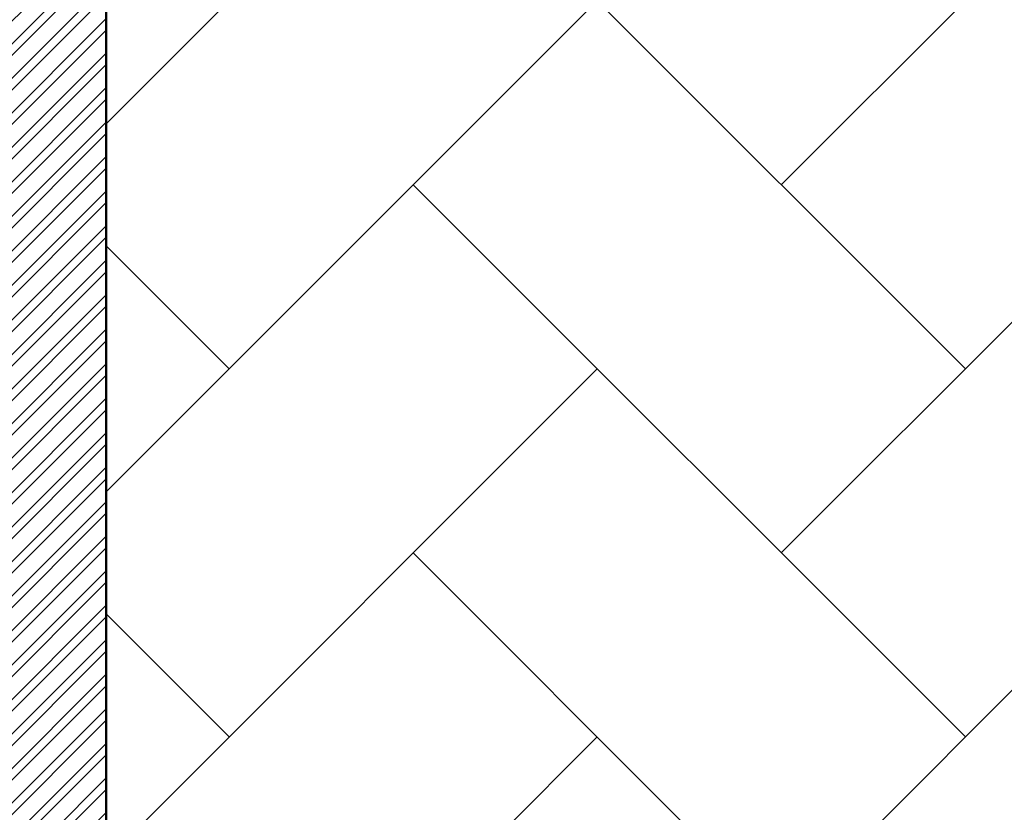
# Model space of a CAD drawing. Units: inches. Extents: x 3590 to 5167, y 65 to 1917.
# Tile 36 of 100: x 4927 to 5003, y 1388 to 1450. Entities that reach past the tile are written whole.
import ezdxf

# ---------------------------------------------------------------- set-up
doc = ezdxf.new("R2010")
doc.units = ezdxf.units.IN
for name, color, linetype, lineweight in [('A-FLOR-PATT', 8, 'Continuous', 13), ('A-WALL', 7, 'Continuous', 50), ('A-WALL-PATT', 251, 'Continuous', 13)]:
    doc.layers.add(name, color=color, linetype=linetype, lineweight=lineweight)

msp = doc.modelspace()

# ---------------------------------------------------------------- hatches: boundary and pattern name
at = {"layer": 'A-FLOR-PATT', "transparency": 33554687}
h = msp.add_hatch(dxfattribs=at)
h.set_pattern_fill('AR-HBONE', color=256, scale=0.2)
h.set_pattern_definition([(45, (-588.972, 0), (0, 28.73682), [60.96, -20.32]), (135, (-574.604, 14.368), (3e-15, 28.73682), [60.96, -20.32])])
h.paths.add_polyline_path([(5071.274, 1796.999), (4933.274, 1796.999), (4933.274, 1753.999), (4962.774, 1753.999, -0.414214), (4928.774, 1719.999), (4933.274, 1718.999), (4933.274, 1334.999), (5071.274, 1334.999)])
h.paths.add_polyline_path([(4951.78, 1521.077), (4951.715, 1521.04), (4951.563, 1520.895)], flags=16)
h.paths.add_polyline_path([(4952.267, 1521.376), (4952.198, 1521.371), (4952.198, 1521.356)], flags=0)
h.paths.add_polyline_path([(4967.051, 1529.728), (4965.231, 1528.694), (4963.411, 1527.714), (4961.756, 1526.851), (4963.589, 1527.449), (4964.036, 1527.478), (4962.975, 1527.249), (4961.76, 1526.852), (4959.792, 1525.834), (4958.005, 1524.895), (4956.24, 1523.93), (4954.504, 1522.919), (4954.129, 1522.682), (4953.361, 1521.997), (4953.366, 1521.998), (4953.605, 1522.064), (4955.106, 1522.761), (4956.921, 1523.434), (4958.678, 1523.915), (4960.358, 1524.2), (4961.945, 1524.286), (4964.171, 1524.108), (4965.958, 1523.309), (4963.863, 1522.976), (4965.187, 1522.499), (4963.366, 1522.497), (4961.545, 1522.487), (4959.764, 1522.461), (4958.304, 1522.419), (4957.974, 1522.388), (4956.307, 1522.232), (4954.718, 1522.071), (4953.251, 1521.899), (4953.525, 1521.623), (4954.331, 1521.379), (4956.243, 1521.23), (4958.039, 1520.93), (4959.684, 1520.483), (4961.16, 1519.896), (4963.107, 1518.8), (4964.393, 1517.325), (4962.973, 1517.726), (4964.558, 1516.661), (4965.407, 1515.708), (4963.507, 1516.322), (4961.68, 1517.005), (4959.935, 1517.745), (4958.282, 1518.528), (4956.732, 1519.343), (4955.295, 1520.175), (4954.672, 1520.572), (4954.513, 1520.627), (4955.658, 1519.318), (4956.703, 1517.982), (4957.644, 1516.647), (4958.485, 1515.334), (4959.55, 1513.524), (4960.438, 1511.769), (4958.841, 1513.62), (4957.452, 1515.325), (4955.819, 1517.459), (4956.665, 1515.448), (4957.111, 1513.923), (4957.447, 1511.714), (4957.076, 1509.793), (4956.538, 1511.11), (4955.992, 1512.569), (4955.444, 1514.125), (4954.898, 1515.735), (4954.357, 1517.356), (4953.824, 1518.943), (4953.305, 1520.452), (4953.065, 1521.116), (4952.971, 1521.146), (4952.949, 1521.086), (4952.73, 1520.199), (4953.37, 1518.024), (4953.757, 1516.373), (4954.051, 1514.765), (4954.264, 1513.221), (4954.471, 1511.131), (4954.497, 1510.402), (4954.409, 1511.76), (4954.264, 1513.221), (4954.051, 1514.765), (4953.757, 1516.373), (4953.37, 1518.024), (4952.877, 1519.698), (4952.716, 1520.141), (4952.533, 1519.059), (4952.374, 1517.789), (4952.219, 1516.312), (4952.046, 1514.6), (4951.833, 1512.626), (4951.557, 1510.363), (4951.203, 1512.168), (4950.852, 1514.339), (4950.985, 1516.376), (4951.66, 1518.286), (4952.593, 1520.481), (4952.357, 1521.13), (4951.855, 1520.328), (4950.839, 1518.908), (4949.777, 1517.587), (4948.916, 1516.617), (4948.111, 1515.256), (4947.089, 1513.554), (4945.889, 1511.615), (4946.326, 1513.402), (4946.562, 1514.249), (4945.528, 1513.327), (4944.581, 1512.531), (4946.018, 1514.508), (4947.204, 1516.048), (4947.893, 1517.313), (4949.307, 1518.764), (4950.414, 1519.767), (4950.451, 1519.806), (4952.267, 1521.376), (4951.645, 1521.493), (4950.404, 1521.18), (4948.044, 1520.359), (4946.119, 1519.452), (4944.572, 1518.475), (4943.35, 1517.443), (4941.997, 1515.92), (4941.661, 1515.275), (4942.813, 1516.99), (4944.572, 1518.475), (4946.119, 1519.452), (4948.044, 1520.359), (4950.404, 1521.18), (4951.645, 1521.493), (4949.647, 1521.868), (4948.6, 1521.756), (4947.126, 1521.57), (4945.42, 1521.348), (4943.45, 1521.105), (4941.183, 1520.856), (4942.86, 1521.613), (4943.873, 1522.03), (4942.952, 1521.909), (4941.41, 1521.485), (4939.543, 1520.67), (4938.968, 1520.226), (4940.733, 1521.299), (4942.952, 1521.909), (4943.702, 1522.008), (4945.894, 1522.7), (4947.565, 1522.714), (4948.921, 1522.566), (4951.131, 1522.183), (4950.971, 1522.297), (4948.129, 1523.006), (4946.035, 1523.707), (4944.232, 1524.521), (4942.707, 1525.461), (4941.444, 1526.537), (4940.43, 1527.761), (4939.649, 1529.143), (4941.421, 1528.122), (4943.147, 1527.132), (4944.841, 1526.175), (4946.514, 1525.25), (4948.179, 1524.359), (4948.365, 1524.263), (4946.475, 1526.045), (4945.181, 1527.54), (4944.19, 1529.033), (4943.496, 1530.54), (4943.278, 1531.36), (4942.498, 1531.919), (4943.114, 1531.762), (4942.959, 1533.659), (4944.14, 1531.989), (4944.612, 1531.323), (4946.202, 1530.463), (4947.486, 1529.509), (4948.79, 1528.226), (4950.368, 1526.237), (4949.485, 1528.155), (4948.851, 1530.123), (4948.491, 1532.041), (4948.381, 1533.918), (4948.501, 1535.76), (4948.827, 1537.573), (4949.418, 1535.565), (4949.957, 1533.569), (4950.464, 1531.586), (4950.961, 1529.617), (4951.391, 1527.954), (4951.724, 1530.687), (4952.201, 1532.58), (4952.889, 1534.33), (4953.77, 1535.951), (4954.827, 1537.46), (4954.521, 1535.39), (4954.273, 1533.937), (4955.58, 1535.663), (4956.748, 1536.739), (4956.159, 1534.78), (4955.589, 1532.873), (4955.043, 1531.006), (4954.525, 1529.166), (4954.038, 1527.341), (4953.638, 1525.733), (4953.611, 1525.586), (4953.398, 1524.166), (4953.382, 1524.009), (4954.07, 1525.476), (4954.912, 1527.022), (4956.136, 1528.894), (4957.847, 1530.577), (4959.376, 1531.54), (4958.256, 1530.104), (4957.143, 1528.663), (4956.066, 1527.243), (4955.056, 1525.871), (4954.141, 1524.571), (4953.352, 1523.372), (4953.311, 1523.303), (4953.273, 1522.925), (4953.261, 1522.382), (4954.103, 1523.373), (4954.63, 1524.284), (4955.961, 1526.358), (4957.23, 1528.13), (4958.421, 1529.609), (4960.037, 1531.368), (4961.374, 1532.375), (4962.101, 1532.77), (4961.07, 1531.061), (4959.987, 1529.438), (4958.869, 1527.908), (4958.15, 1527.007), (4959.803, 1528.003), (4961.589, 1528.793), (4963.391, 1529.328), (4965.211, 1529.632)], flags=16)
h.paths.add_polyline_path([(4962.944, 1523.182), (4961.107, 1523.422), (4960.392, 1523.362), (4962.35, 1523.331)], flags=0)
h.paths.add_polyline_path([(5049.541, 1584.551), (5049.476, 1584.515), (5049.325, 1584.37)], flags=16)
h.paths.add_polyline_path([(5050.028, 1584.851), (5049.959, 1584.845), (5049.959, 1584.83)], flags=0)
h.paths.add_polyline_path([(5042.333, 1581.949), (5043.88, 1582.926), (5045.806, 1583.833), (5048.165, 1584.654), (5049.406, 1584.967), (5047.408, 1585.342), (5046.361, 1585.231), (5044.888, 1585.044), (5043.181, 1584.822), (5041.211, 1584.579), (5038.944, 1584.33), (5040.622, 1585.087), (5041.634, 1585.504), (5040.713, 1585.383), (5039.171, 1584.959), (5037.304, 1584.144), (5036.729, 1583.7), (5038.494, 1584.773), (5040.713, 1585.383), (5041.463, 1585.482), (5043.655, 1586.174), (5045.326, 1586.188), (5046.682, 1586.04), (5048.893, 1585.657), (5048.732, 1585.771), (5045.891, 1586.48), (5043.796, 1587.181), (5041.994, 1587.996), (5040.468, 1588.935), (5039.205, 1590.011), (5038.191, 1591.235), (5037.41, 1592.617), (5039.182, 1591.596), (5040.909, 1590.607), (5042.602, 1589.649), (5044.275, 1588.724), (5045.94, 1587.833), (5046.126, 1587.738), (5044.237, 1589.519), (5042.942, 1591.015), (5041.952, 1592.508), (5041.257, 1594.014), (5041.039, 1594.834), (5040.26, 1595.393), (5040.875, 1595.237), (5040.721, 1597.133), (5041.901, 1595.463), (5042.373, 1594.798), (5043.963, 1593.938), (5045.247, 1592.983), (5046.552, 1591.701), (5048.129, 1589.712), (5047.247, 1591.63), (5046.613, 1593.597), (5046.252, 1595.515), (5046.142, 1597.392), (5046.262, 1599.234), (5046.588, 1601.047), (5047.179, 1599.039), (5047.718, 1597.043), (5048.225, 1595.06), (5048.722, 1593.091), (5049.152, 1591.429), (5049.485, 1594.161), (5049.962, 1596.054), (5050.65, 1597.804), (5051.532, 1599.425), (5052.589, 1600.934), (5052.283, 1598.864), (5052.034, 1597.411), (5053.341, 1599.137), (5054.509, 1600.213), (5053.92, 1598.254), (5053.35, 1596.348), (5052.805, 1594.48), (5052.286, 1592.64), (5051.799, 1590.815), (5051.4, 1589.207), (5051.373, 1589.06), (5051.159, 1587.64), (5051.143, 1587.483), (5051.831, 1588.95), (5052.673, 1590.496), (5053.898, 1592.368), (5055.608, 1594.051), (5057.137, 1595.014), (5056.017, 1593.578), (5054.904, 1592.137), (5053.828, 1590.717), (5052.817, 1589.345), (5051.902, 1588.046), (5051.113, 1586.846), (5051.072, 1586.777), (5051.034, 1586.399), (5051.022, 1585.856), (5051.864, 1586.847), (5052.391, 1587.758), (5053.723, 1589.832), (5054.991, 1591.604), (5056.182, 1593.083), (5057.798, 1594.842), (5059.135, 1595.849), (5059.863, 1596.244), (5058.831, 1594.535), (5057.749, 1592.912), (5056.63, 1591.382), (5055.912, 1590.482), (5057.564, 1591.477), (5059.35, 1592.267), (5061.152, 1592.802), (5062.972, 1593.106), (5064.812, 1593.203), (5062.992, 1592.169), (5061.172, 1591.188), (5059.518, 1590.325), (5061.35, 1590.924), (5061.797, 1590.952), (5060.737, 1590.723), (5059.521, 1590.326), (5057.553, 1589.308), (5055.766, 1588.369), (5054.002, 1587.404), (5052.265, 1586.393), (5051.891, 1586.156), (5051.122, 1585.471), (5051.127, 1585.472), (5051.366, 1585.538), (5052.867, 1586.235), (5054.682, 1586.908), (5056.439, 1587.389), (5058.12, 1587.675), (5059.706, 1587.76), (5061.933, 1587.583), (5063.719, 1586.783), (5061.624, 1586.45), (5062.949, 1585.973), (5061.127, 1585.971), (5059.307, 1585.961), (5057.525, 1585.935), (5056.065, 1585.893), (5055.735, 1585.862), (5054.068, 1585.707), (5052.479, 1585.546), (5051.012, 1585.373), (5051.286, 1585.097), (5052.092, 1584.853), (5054.004, 1584.704), (5055.8, 1584.404), (5057.446, 1583.958), (5058.921, 1583.37), (5060.868, 1582.274), (5062.154, 1580.799), (5060.734, 1581.2), (5062.32, 1580.135), (5063.168, 1579.182), (5061.269, 1579.796), (5059.441, 1580.479), (5057.696, 1581.219), (5056.043, 1582.003), (5054.493, 1582.817), (5053.057, 1583.649), (5052.433, 1584.047), (5052.274, 1584.101), (5053.42, 1582.793), (5054.464, 1581.457), (5055.405, 1580.121), (5056.247, 1578.809), (5057.311, 1576.998), (5058.199, 1575.244), (5056.602, 1577.094), (5055.213, 1578.799), (5053.58, 1580.933), (5054.427, 1578.922), (5054.872, 1577.397), (5055.208, 1575.189), (5054.838, 1573.267), (5054.299, 1574.584), (5053.754, 1576.043), (5053.206, 1577.599), (5052.659, 1579.209), (5052.118, 1580.83), (5051.585, 1582.417), (5051.066, 1583.927), (5050.826, 1584.59), (5050.733, 1584.62), (5050.711, 1584.561), (5050.491, 1583.673), (5051.131, 1581.498), (5051.518, 1579.847), (5051.813, 1578.24), (5052.026, 1576.695), (5052.233, 1574.605), (5052.258, 1573.876), (5052.17, 1575.234), (5052.026, 1576.695), (5051.813, 1578.24), (5051.518, 1579.847), (5051.131, 1581.498), (5050.638, 1583.172), (5050.477, 1583.615), (5050.294, 1582.533), (5050.136, 1581.263), (5049.981, 1579.786), (5049.807, 1578.074), (5049.594, 1576.1), (5049.318, 1573.837), (5048.965, 1575.642), (5048.613, 1577.813), (5048.747, 1579.85), (5049.421, 1581.76), (5050.354, 1583.955), (5050.118, 1584.604), (5049.616, 1583.802), (5048.6, 1582.382), (5047.538, 1581.061), (5046.677, 1580.091), (5045.872, 1578.73), (5044.85, 1577.028), (5043.651, 1575.089), (5044.087, 1576.877), (5044.324, 1577.723), (5043.289, 1576.801), (5042.342, 1576.005), (5043.779, 1577.982), (5044.966, 1579.522), (5045.655, 1580.787), (5047.068, 1582.239), (5048.175, 1583.241), (5048.213, 1583.28), (5050.028, 1584.851), (5049.406, 1584.967), (5048.165, 1584.654), (5045.806, 1583.833), (5043.88, 1582.926), (5042.333, 1581.949), (5041.111, 1580.917), (5039.758, 1579.394), (5039.423, 1578.749), (5040.575, 1580.464)], flags=16)
h.paths.add_polyline_path([(4954.799, 1533.12), (4954.262, 1532.079), (4953.831, 1530.935), (4953.505, 1529.636), (4953.283, 1528.133), (4953.167, 1526.376), (4953.156, 1524.315), (4953.277, 1521.236), (4952.802, 1521.842), (4951.557, 1521.998), (4950.976, 1521.961), (4952.661, 1521.941), (4952.802, 1521.842), (4953.152, 1523.593), (4953.167, 1526.376), (4953.283, 1528.133), (4953.609, 1530.346), (4954.456, 1532.592)], flags=0)
h.paths.add_polyline_path([(5050.563, 1585.316), (5049.318, 1585.472), (5048.737, 1585.435), (5050.422, 1585.415), (5050.563, 1585.316), (5050.914, 1587.067), (5050.928, 1589.851), (5051.045, 1591.607), (5051.371, 1593.82), (5052.217, 1596.066), (5052.56, 1596.594), (5052.024, 1595.554), (5051.592, 1594.409), (5051.266, 1593.11), (5051.045, 1591.607), (5050.928, 1589.851), (5050.918, 1587.789), (5051.038, 1584.71)], flags=0)
h.paths.add_polyline_path([(5058.153, 1586.836), (5060.111, 1586.805), (5060.705, 1586.656), (5058.868, 1586.896)], flags=0)
h.paths.add_polyline_path([(5049.541, 1430.936), (5049.476, 1430.9), (5049.325, 1430.755)], flags=16)
h.paths.add_polyline_path([(5050.028, 1431.236), (5049.959, 1431.231), (5049.959, 1431.215)], flags=0)
h.paths.add_polyline_path([(5046.588, 1447.432), (5047.179, 1445.425), (5047.718, 1443.429), (5048.225, 1441.446), (5048.722, 1439.476), (5049.152, 1437.814), (5049.485, 1440.546), (5049.962, 1442.439), (5050.65, 1444.189), (5051.532, 1445.811), (5052.589, 1447.319), (5052.283, 1445.249), (5052.034, 1443.796), (5053.341, 1445.522), (5054.509, 1446.598), (5053.92, 1444.64), (5053.35, 1442.733), (5052.805, 1440.865), (5052.286, 1439.025), (5051.799, 1437.201), (5051.4, 1435.592), (5051.373, 1435.445), (5051.159, 1434.025), (5051.143, 1433.868), (5051.831, 1435.335), (5052.673, 1436.881), (5053.898, 1438.753), (5055.608, 1440.436), (5057.137, 1441.4), (5056.017, 1439.963), (5054.904, 1438.522), (5053.828, 1437.102), (5052.817, 1435.73), (5051.902, 1434.431), (5051.113, 1433.231), (5051.072, 1433.162), (5051.034, 1432.784), (5051.022, 1432.242), (5051.864, 1433.232), (5052.391, 1434.143), (5053.723, 1436.217), (5054.991, 1437.989), (5056.182, 1439.468), (5057.798, 1441.227), (5059.135, 1442.235), (5059.863, 1442.629), (5058.831, 1440.921), (5057.749, 1439.298), (5056.63, 1437.767), (5055.912, 1436.867), (5057.564, 1437.863), (5059.35, 1438.652), (5061.152, 1439.187), (5062.972, 1439.491), (5064.812, 1439.588), (5062.992, 1438.554), (5061.172, 1437.573), (5059.518, 1436.71), (5061.35, 1437.309), (5061.797, 1437.337), (5060.737, 1437.108), (5059.521, 1436.711), (5057.553, 1435.693), (5055.766, 1434.754), (5054.002, 1433.789), (5052.265, 1432.778), (5051.891, 1432.541), (5051.122, 1431.856), (5051.127, 1431.857), (5051.366, 1431.923), (5052.867, 1432.62), (5054.682, 1433.293), (5056.439, 1433.775), (5058.12, 1434.06), (5059.706, 1434.145), (5061.933, 1433.968), (5063.719, 1433.168), (5061.624, 1432.835), (5062.949, 1432.358), (5061.127, 1432.357), (5059.307, 1432.346), (5057.525, 1432.32), (5056.065, 1432.278), (5055.735, 1432.248), (5054.068, 1432.092), (5052.479, 1431.931), (5051.012, 1431.759), (5051.286, 1431.482), (5052.092, 1431.238), (5054.004, 1431.089), (5055.8, 1430.789), (5057.446, 1430.343), (5058.921, 1429.755), (5060.868, 1428.66), (5062.154, 1427.185), (5060.734, 1427.585), (5062.32, 1426.52), (5063.168, 1425.567), (5061.269, 1426.181), (5059.441, 1426.865), (5057.696, 1427.604), (5056.043, 1428.388), (5054.493, 1429.202), (5053.057, 1430.034), (5052.433, 1430.432), (5052.274, 1430.487), (5053.42, 1429.178), (5054.464, 1427.842), (5055.405, 1426.506), (5056.247, 1425.194), (5057.311, 1423.383), (5058.199, 1421.629), (5056.602, 1423.479), (5055.213, 1425.184), (5053.58, 1427.318), (5054.427, 1425.307), (5054.872, 1423.782), (5055.208, 1421.574), (5054.838, 1419.652), (5054.299, 1420.97), (5053.754, 1422.428), (5053.206, 1423.984), (5052.659, 1425.595), (5052.118, 1427.215), (5051.585, 1428.802), (5051.066, 1430.312), (5050.826, 1430.975), (5050.733, 1431.005), (5050.711, 1430.946), (5050.491, 1430.058), (5051.131, 1427.883), (5051.518, 1426.232), (5051.813, 1424.625), (5052.026, 1423.081), (5052.233, 1420.991), (5052.258, 1420.261), (5052.17, 1421.619), (5052.026, 1423.081), (5051.813, 1424.625), (5051.518, 1426.232), (5051.131, 1427.883), (5050.638, 1429.558), (5050.477, 1430.001), (5050.294, 1428.918), (5050.136, 1427.648), (5049.981, 1426.171), (5049.807, 1424.459), (5049.594, 1422.485), (5049.318, 1420.222), (5048.965, 1422.028), (5048.613, 1424.199), (5048.747, 1426.235), (5049.421, 1428.146), (5050.354, 1430.34), (5050.118, 1430.989), (5049.616, 1430.187), (5048.6, 1428.768), (5047.538, 1427.446), (5046.677, 1426.477), (5045.872, 1425.116), (5044.85, 1423.413), (5043.651, 1421.474), (5044.087, 1423.262), (5044.324, 1424.109), (5043.289, 1423.186), (5042.342, 1422.391), (5043.779, 1424.368), (5044.966, 1425.907), (5045.655, 1427.173), (5047.068, 1428.624), (5048.175, 1429.627), (5048.213, 1429.666), (5050.028, 1431.236), (5049.406, 1431.353), (5048.165, 1431.039), (5045.806, 1430.218), (5043.88, 1429.311), (5042.333, 1428.334), (5041.111, 1427.302), (5039.758, 1425.779), (5039.423, 1425.134), (5040.575, 1426.849), (5042.333, 1428.334), (5043.88, 1429.311), (5045.806, 1430.218), (5048.165, 1431.039), (5049.406, 1431.353), (5047.408, 1431.727), (5046.361, 1431.616), (5044.888, 1431.429), (5043.181, 1431.207), (5041.211, 1430.964), (5038.944, 1430.715), (5040.622, 1431.472), (5041.634, 1431.89), (5040.713, 1431.769), (5039.171, 1431.345), (5037.304, 1430.53), (5036.729, 1430.085), (5038.494, 1431.158), (5040.713, 1431.769), (5041.463, 1431.867), (5043.655, 1432.559), (5045.326, 1432.573), (5046.682, 1432.425), (5048.893, 1432.042), (5048.732, 1432.156), (5045.891, 1432.865), (5043.796, 1433.566), (5041.994, 1434.381), (5040.468, 1435.321), (5039.205, 1436.396), (5038.191, 1437.62), (5037.41, 1439.002), (5039.182, 1437.982), (5040.909, 1436.992), (5042.602, 1436.034), (5044.275, 1435.109), (5045.94, 1434.218), (5046.126, 1434.123), (5044.237, 1435.904), (5042.942, 1437.4), (5041.952, 1438.893), (5041.257, 1440.399), (5041.039, 1441.219), (5040.26, 1441.778), (5040.875, 1441.622), (5040.721, 1443.518), (5041.901, 1441.848), (5042.373, 1441.183), (5043.963, 1440.323), (5045.247, 1439.369), (5046.552, 1438.086), (5048.129, 1436.097), (5047.247, 1438.015), (5046.613, 1439.982), (5046.252, 1441.901), (5046.142, 1443.778), (5046.262, 1445.619)], flags=16)
h.paths.add_polyline_path([(5052.382, 1444.255), (5051.623, 1442.78), (5052.024, 1441.939), (5052.56, 1442.98)], flags=0)
h.paths.add_polyline_path([(5050.563, 1431.701), (5049.318, 1431.857), (5048.737, 1431.821), (5050.422, 1431.8)], flags=0)
h.paths.add_polyline_path([(5058.153, 1433.221), (5060.111, 1433.19), (5060.705, 1433.041), (5058.868, 1433.281)], flags=0)
h.paths.add_polyline_path([(5049.541, 1352.285), (5049.476, 1352.249), (5049.325, 1352.104)], flags=16)
h.paths.add_polyline_path([(5050.028, 1352.585), (5049.959, 1352.58), (5049.959, 1352.564)], flags=0)
h.paths.add_polyline_path([(5046.588, 1368.781), (5047.179, 1366.774), (5047.718, 1364.778), (5048.225, 1362.795), (5048.722, 1360.825), (5049.152, 1359.163), (5049.485, 1361.896), (5049.962, 1363.789), (5050.65, 1365.538), (5051.532, 1367.16), (5052.589, 1368.669), (5052.283, 1366.598), (5052.034, 1365.145), (5053.341, 1366.871), (5054.509, 1367.947), (5053.92, 1365.989), (5053.35, 1364.082), (5052.805, 1362.214), (5052.286, 1360.374), (5051.799, 1358.55), (5051.4, 1356.942), (5051.373, 1356.794), (5051.159, 1355.374), (5051.143, 1355.218), (5051.831, 1356.684), (5052.673, 1358.23), (5053.898, 1360.102), (5055.608, 1361.786), (5057.137, 1362.749), (5056.017, 1361.313), (5054.904, 1359.872), (5053.828, 1358.452), (5052.817, 1357.079), (5051.902, 1355.78), (5051.113, 1354.581), (5051.072, 1354.512), (5051.034, 1354.133), (5051.022, 1353.591), (5051.864, 1354.581), (5052.391, 1355.492), (5053.723, 1357.566), (5054.991, 1359.338), (5056.182, 1360.817), (5057.798, 1362.577), (5059.135, 1363.584), (5059.863, 1363.979), (5058.831, 1362.27), (5057.749, 1360.647), (5056.63, 1359.117), (5055.912, 1358.216), (5057.564, 1359.212), (5059.35, 1360.001), (5061.152, 1360.536), (5062.972, 1360.841), (5064.812, 1360.937), (5062.992, 1359.903), (5061.172, 1358.923), (5059.518, 1358.059), (5061.35, 1358.658), (5061.797, 1358.687), (5060.737, 1358.458), (5059.521, 1358.061), (5057.553, 1357.043), (5055.766, 1356.103), (5054.002, 1355.138), (5052.265, 1354.127), (5051.891, 1353.89), (5051.122, 1353.206), (5051.127, 1353.206), (5051.366, 1353.272), (5052.867, 1353.969), (5054.682, 1354.643), (5056.439, 1355.124), (5058.12, 1355.409), (5059.706, 1355.495), (5061.933, 1355.317), (5063.719, 1354.518), (5061.624, 1354.184), (5062.949, 1353.708), (5061.127, 1353.706), (5059.307, 1353.695), (5057.525, 1353.669), (5056.065, 1353.627), (5055.735, 1353.597), (5054.068, 1353.441), (5052.479, 1353.28), (5051.012, 1353.108), (5051.286, 1352.831), (5052.092, 1352.587), (5054.004, 1352.439), (5055.8, 1352.138), (5057.446, 1351.692), (5058.921, 1351.104), (5060.868, 1350.009), (5062.154, 1348.534), (5060.734, 1348.935), (5062.32, 1347.869), (5063.168, 1346.916), (5061.269, 1347.53), (5059.441, 1348.214), (5057.696, 1348.954), (5056.043, 1349.737), (5054.493, 1350.551), (5053.057, 1351.383), (5052.433, 1351.781), (5052.274, 1351.836), (5053.42, 1350.527), (5054.464, 1349.191), (5055.405, 1347.855), (5056.247, 1346.543), (5057.311, 1344.733), (5058.199, 1342.978), (5056.602, 1344.828), (5055.213, 1346.534), (5053.58, 1348.667), (5054.427, 1346.656), (5054.872, 1345.132), (5055.208, 1342.923), (5054.838, 1341.002), (5054.299, 1342.319), (5053.754, 1343.778), (5053.206, 1345.334), (5052.659, 1346.944), (5052.118, 1348.564), (5051.585, 1350.151), (5051.066, 1351.661), (5050.826, 1352.324), (5050.733, 1352.355), (5050.711, 1352.295), (5050.491, 1351.408), (5051.131, 1349.232), (5051.518, 1347.581), (5051.813, 1345.974), (5052.026, 1344.43), (5052.233, 1342.34), (5052.258, 1341.61), (5052.17, 1342.969), (5052.026, 1344.43), (5051.813, 1345.974), (5051.518, 1347.581), (5051.131, 1349.232), (5050.638, 1350.907), (5050.477, 1351.35), (5050.294, 1350.267), (5050.136, 1348.997), (5049.981, 1347.52), (5049.807, 1345.809), (5049.594, 1343.835), (5049.318, 1341.571), (5048.965, 1343.377), (5048.613, 1345.548), (5048.747, 1347.585), (5049.421, 1349.495), (5050.354, 1351.689), (5050.118, 1352.339), (5049.616, 1351.536), (5048.6, 1350.117), (5047.538, 1348.795), (5046.677, 1347.826), (5045.872, 1346.465), (5044.85, 1344.763), (5043.651, 1342.824), (5044.087, 1344.611), (5044.324, 1345.458), (5043.289, 1344.535), (5042.342, 1343.74), (5043.779, 1345.717), (5044.966, 1347.256), (5045.655, 1348.522), (5047.068, 1349.973), (5048.175, 1350.976), (5048.213, 1351.015), (5050.028, 1352.585), (5049.406, 1352.702), (5048.165, 1352.388), (5045.806, 1351.567), (5043.88, 1350.661), (5042.333, 1349.683), (5041.111, 1348.651), (5039.758, 1347.128), (5039.423, 1346.483), (5040.575, 1348.198), (5042.333, 1349.683), (5043.88, 1350.661), (5045.806, 1351.567), (5048.165, 1352.388), (5049.406, 1352.702), (5047.408, 1353.076), (5046.361, 1352.965), (5044.888, 1352.779), (5043.181, 1352.556), (5041.211, 1352.313), (5038.944, 1352.065), (5040.622, 1352.821), (5041.634, 1353.239), (5040.713, 1353.118), (5039.171, 1352.694), (5037.304, 1351.879), (5036.729, 1351.434), (5038.494, 1352.508), (5040.713, 1353.118), (5041.463, 1353.216), (5043.655, 1353.909), (5045.326, 1353.923), (5046.682, 1353.774), (5048.893, 1353.391), (5048.732, 1353.506), (5045.891, 1354.214), (5043.796, 1354.915), (5041.994, 1355.73), (5040.468, 1356.67), (5039.205, 1357.746), (5038.191, 1358.969), (5037.41, 1360.352), (5039.182, 1359.331), (5040.909, 1358.341), (5042.602, 1357.383), (5044.275, 1356.458), (5045.94, 1355.567), (5046.126, 1355.472), (5044.237, 1357.253), (5042.942, 1358.749), (5041.952, 1360.242), (5041.257, 1361.748), (5041.039, 1362.568), (5040.26, 1363.128), (5040.875, 1362.971), (5040.721, 1364.867), (5041.901, 1363.197), (5042.373, 1362.532), (5043.963, 1361.672), (5045.247, 1360.718), (5046.552, 1359.435), (5048.129, 1357.446), (5047.247, 1359.364), (5046.613, 1361.331), (5046.252, 1363.25), (5046.142, 1365.127), (5046.262, 1366.969)], flags=16)
h.paths.add_polyline_path([(5052.382, 1365.604), (5051.623, 1364.129), (5052.024, 1363.288), (5052.56, 1364.329)], flags=0)
h.paths.add_polyline_path([(4951.78, 1698.041), (4951.715, 1698.005), (4951.563, 1697.859)], flags=16)
h.paths.add_polyline_path([(4952.267, 1698.341), (4952.198, 1698.335), (4952.198, 1698.32)], flags=0)
h.paths.add_polyline_path([(4957.076, 1686.757), (4956.538, 1688.074), (4955.992, 1689.533), (4955.444, 1691.089), (4954.898, 1692.699), (4954.357, 1694.32), (4953.824, 1695.907), (4953.305, 1697.417), (4953.065, 1698.08), (4952.971, 1698.11), (4952.949, 1698.051), (4952.73, 1697.163), (4953.37, 1694.988), (4953.757, 1693.337), (4954.051, 1691.729), (4954.264, 1690.185), (4954.471, 1688.095), (4954.497, 1687.366), (4954.409, 1688.724), (4954.264, 1690.185), (4954.051, 1691.729), (4953.757, 1693.337), (4953.37, 1694.988), (4952.877, 1696.662), (4952.716, 1697.105), (4952.533, 1696.023), (4952.374, 1694.753), (4952.219, 1693.276), (4952.046, 1691.564), (4951.833, 1689.59), (4951.557, 1687.327), (4951.203, 1689.132), (4950.852, 1691.303), (4950.985, 1693.34), (4951.66, 1695.25), (4952.593, 1697.445), (4952.357, 1698.094), (4951.855, 1697.292), (4950.839, 1695.872), (4949.777, 1694.551), (4948.916, 1693.581), (4948.111, 1692.22), (4947.089, 1690.518), (4945.889, 1688.579), (4946.326, 1690.366), (4946.562, 1691.213), (4945.528, 1690.291), (4944.581, 1689.495), (4946.018, 1691.472), (4947.204, 1693.012), (4947.893, 1694.277), (4949.307, 1695.729), (4950.414, 1696.731), (4950.451, 1696.77), (4952.267, 1698.341), (4951.645, 1698.457), (4950.404, 1698.144), (4948.044, 1697.323), (4946.119, 1696.416), (4944.572, 1695.439), (4943.35, 1694.407), (4941.997, 1692.884), (4941.661, 1692.239), (4942.813, 1693.954), (4944.572, 1695.439), (4946.119, 1696.416), (4948.044, 1697.323), (4950.404, 1698.144), (4951.645, 1698.457), (4949.647, 1698.832), (4948.6, 1698.72), (4947.126, 1698.534), (4945.42, 1698.312), (4943.45, 1698.069), (4941.183, 1697.82), (4942.86, 1698.577), (4943.873, 1698.994), (4942.952, 1698.873), (4941.41, 1698.449), (4939.543, 1697.634), (4938.968, 1697.19), (4940.733, 1698.263), (4942.952, 1698.873), (4943.702, 1698.972), (4945.894, 1699.664), (4947.565, 1699.678), (4948.921, 1699.53), (4951.131, 1699.147), (4950.971, 1699.261), (4948.129, 1699.97), (4946.035, 1700.671), (4944.232, 1701.486), (4942.707, 1702.425), (4941.444, 1703.501), (4940.43, 1704.725), (4939.649, 1706.107), (4941.421, 1705.086), (4943.147, 1704.097), (4944.841, 1703.139), (4946.514, 1702.214), (4948.179, 1701.323), (4948.365, 1701.227), (4946.475, 1703.009), (4945.181, 1704.505), (4944.19, 1705.997), (4943.496, 1707.504), (4943.278, 1708.324), (4942.498, 1708.883), (4943.114, 1708.727), (4942.959, 1710.623), (4944.14, 1708.953), (4944.612, 1708.287), (4946.202, 1707.428), (4947.486, 1706.473), (4948.79, 1705.191), (4950.368, 1703.202), (4949.485, 1705.12), (4948.851, 1707.087), (4948.491, 1709.005), (4948.381, 1710.882), (4948.501, 1712.724), (4948.827, 1714.537), (4949.418, 1712.529), (4949.957, 1710.533), (4950.464, 1708.55), (4950.961, 1706.581), (4951.391, 1704.919), (4951.724, 1707.651), (4952.201, 1709.544), (4952.889, 1711.294), (4953.77, 1712.915), (4954.827, 1714.424), (4954.521, 1712.354), (4954.273, 1710.901), (4955.58, 1712.627), (4956.748, 1713.703), (4956.159, 1711.744), (4955.589, 1709.837), (4955.043, 1707.97), (4954.525, 1706.13), (4954.038, 1704.305), (4953.638, 1702.697), (4953.611, 1702.55), (4953.398, 1701.13), (4953.382, 1700.973), (4954.07, 1702.44), (4954.912, 1703.986), (4956.136, 1705.858), (4957.847, 1707.541), (4959.376, 1708.504), (4958.256, 1707.068), (4957.143, 1705.627), (4956.066, 1704.207), (4955.056, 1702.835), (4954.141, 1701.536), (4953.352, 1700.336), (4953.311, 1700.267), (4953.273, 1699.889), (4953.261, 1699.346), (4954.103, 1700.337), (4954.63, 1701.248), (4955.961, 1703.322), (4957.23, 1705.094), (4958.421, 1706.573), (4960.037, 1708.332), (4961.374, 1709.339), (4962.101, 1709.734), (4961.07, 1708.025), (4959.987, 1706.402), (4958.869, 1704.872), (4958.15, 1703.972), (4959.803, 1704.967), (4961.589, 1705.757), (4963.391, 1706.292), (4965.211, 1706.596), (4967.051, 1706.692), (4965.231, 1705.659), (4963.411, 1704.678), (4961.756, 1703.815), (4963.589, 1704.413), (4964.036, 1704.442), (4962.975, 1704.213), (4961.76, 1703.816), (4959.792, 1702.798), (4958.005, 1701.859), (4956.24, 1700.894), (4954.504, 1699.883), (4954.129, 1699.646), (4953.361, 1698.961), (4953.366, 1698.962), (4953.605, 1699.028), (4955.106, 1699.725), (4956.921, 1700.398), (4958.678, 1700.879), (4960.358, 1701.164), (4961.945, 1701.25), (4964.171, 1701.073), (4965.958, 1700.273), (4963.863, 1699.94), (4965.187, 1699.463), (4963.366, 1699.461), (4961.545, 1699.451), (4959.764, 1699.425), (4958.304, 1699.383), (4957.974, 1699.352), (4956.307, 1699.197), (4954.718, 1699.036), (4953.251, 1698.863), (4953.525, 1698.587), (4954.331, 1698.343), (4956.243, 1698.194), (4958.039, 1697.894), (4959.684, 1697.447), (4961.16, 1696.86), (4963.107, 1695.764), (4964.393, 1694.289), (4962.973, 1694.69), (4964.558, 1693.625), (4965.407, 1692.672), (4963.507, 1693.286), (4961.68, 1693.969), (4959.935, 1694.709), (4958.282, 1695.492), (4956.732, 1696.307), (4955.295, 1697.139), (4954.672, 1697.536), (4954.513, 1697.591), (4955.658, 1696.282), (4956.703, 1694.946), (4957.644, 1693.611), (4958.485, 1692.298), (4959.55, 1690.488), (4960.438, 1688.733), (4958.841, 1690.584), (4957.452, 1692.289), (4955.819, 1694.423), (4956.665, 1692.412), (4957.111, 1690.887), (4957.447, 1688.678)], flags=16)
h.paths.add_polyline_path([(5050.563, 1353.05), (5049.318, 1353.207), (5048.737, 1353.17), (5050.422, 1353.15)], flags=0)
h.paths.add_polyline_path([(4951.78, 1351.486), (4951.715, 1351.45), (4951.563, 1351.305)], flags=16)
h.paths.add_polyline_path([(4952.267, 1351.786), (4952.198, 1351.78), (4952.198, 1351.765)], flags=0)
h.paths.add_polyline_path([(4954.827, 1367.869), (4954.521, 1365.799), (4954.273, 1364.346), (4955.58, 1366.072), (4956.748, 1367.148), (4956.159, 1365.19), (4955.589, 1363.283), (4955.043, 1361.415), (4954.525, 1359.575), (4954.038, 1357.751), (4953.638, 1356.142), (4953.611, 1355.995), (4953.398, 1354.575), (4953.382, 1354.418), (4954.07, 1355.885), (4954.912, 1357.431), (4956.136, 1359.303), (4957.847, 1360.986), (4959.376, 1361.95), (4958.256, 1360.513), (4957.143, 1359.072), (4956.066, 1357.652), (4955.056, 1356.28), (4954.141, 1354.981), (4953.352, 1353.781), (4953.311, 1353.712), (4953.273, 1353.334), (4953.261, 1352.792), (4954.103, 1353.782), (4954.63, 1354.693), (4955.961, 1356.767), (4957.23, 1358.539), (4958.421, 1360.018), (4960.037, 1361.777), (4961.374, 1362.785), (4962.101, 1363.179), (4961.07, 1361.471), (4959.987, 1359.848), (4958.869, 1358.317), (4958.15, 1357.417), (4959.803, 1358.413), (4961.589, 1359.202), (4963.391, 1359.737), (4965.211, 1360.041), (4967.051, 1360.138), (4965.231, 1359.104), (4963.411, 1358.123), (4961.756, 1357.26), (4963.589, 1357.859), (4964.036, 1357.887), (4962.975, 1357.658), (4961.76, 1357.261), (4959.792, 1356.243), (4958.005, 1355.304), (4956.24, 1354.339), (4954.504, 1353.328), (4954.129, 1353.091), (4953.361, 1352.406), (4953.366, 1352.407), (4953.605, 1352.473), (4955.106, 1353.17), (4956.921, 1353.843), (4958.678, 1354.325), (4960.358, 1354.61), (4961.945, 1354.695), (4964.171, 1354.518), (4965.958, 1353.718), (4963.863, 1353.385), (4965.187, 1352.908), (4963.366, 1352.907), (4961.545, 1352.896), (4959.764, 1352.87), (4958.304, 1352.828), (4957.974, 1352.798), (4956.307, 1352.642), (4954.718, 1352.481), (4953.251, 1352.309), (4953.525, 1352.032), (4954.331, 1351.788), (4956.243, 1351.639), (4958.039, 1351.339), (4959.684, 1350.893), (4961.16, 1350.305), (4963.107, 1349.21), (4964.393, 1347.735), (4962.973, 1348.135), (4964.558, 1347.07), (4965.407, 1346.117), (4963.507, 1346.731), (4961.68, 1347.414), (4959.935, 1348.154), (4958.282, 1348.938), (4956.732, 1349.752), (4955.295, 1350.584), (4954.672, 1350.982), (4954.513, 1351.036), (4955.658, 1349.728), (4956.703, 1348.392), (4957.644, 1347.056), (4958.485, 1345.744), (4959.55, 1343.933), (4960.438, 1342.179), (4958.841, 1344.029), (4957.452, 1345.734), (4955.819, 1347.868), (4956.665, 1345.857), (4957.111, 1344.332), (4957.447, 1342.124), (4957.076, 1340.202), (4956.538, 1341.52), (4955.992, 1342.978), (4955.444, 1344.534), (4954.898, 1346.145), (4954.357, 1347.765), (4953.824, 1349.352), (4953.305, 1350.862), (4953.065, 1351.525), (4952.971, 1351.555), (4952.949, 1351.496), (4952.73, 1350.608), (4953.37, 1348.433), (4953.757, 1346.782), (4954.051, 1345.175), (4954.264, 1343.631), (4954.471, 1341.541), (4954.497, 1340.811), (4954.409, 1342.169), (4954.264, 1343.631), (4954.051, 1345.175), (4953.757, 1346.782), (4953.37, 1348.433), (4952.877, 1350.108), (4952.716, 1350.551), (4952.533, 1349.468), (4952.374, 1348.198), (4952.219, 1346.721), (4952.046, 1345.009), (4951.833, 1343.035), (4951.557, 1340.772), (4951.203, 1342.578), (4950.852, 1344.749), (4950.985, 1346.785), (4951.66, 1348.696), (4952.593, 1350.89), (4952.357, 1351.539), (4951.855, 1350.737), (4950.839, 1349.318), (4949.777, 1347.996), (4948.916, 1347.027), (4948.111, 1345.665), (4947.089, 1343.963), (4945.889, 1342.024), (4946.326, 1343.812), (4946.562, 1344.659), (4945.528, 1343.736), (4944.581, 1342.941), (4946.018, 1344.918), (4947.204, 1346.457), (4947.893, 1347.723), (4949.307, 1349.174), (4950.414, 1350.177), (4950.451, 1350.216), (4952.267, 1351.786), (4951.645, 1351.903), (4950.404, 1351.589), (4948.044, 1350.768), (4946.119, 1349.861), (4944.572, 1348.884), (4943.35, 1347.852), (4941.997, 1346.329), (4941.661, 1345.684), (4942.813, 1347.399), (4944.572, 1348.884), (4946.119, 1349.861), (4948.044, 1350.768), (4950.404, 1351.589), (4951.645, 1351.903), (4949.647, 1352.277), (4948.6, 1352.166), (4947.126, 1351.979), (4945.42, 1351.757), (4943.45, 1351.514), (4941.183, 1351.265), (4942.86, 1352.022), (4943.873, 1352.44), (4942.952, 1352.319), (4941.41, 1351.895), (4939.543, 1351.08), (4938.968, 1350.635), (4940.733, 1351.708), (4942.952, 1352.319), (4943.702, 1352.417), (4945.894, 1353.109), (4947.565, 1353.123), (4948.921, 1352.975), (4951.131, 1352.592), (4950.971, 1352.706), (4948.129, 1353.415), (4946.035, 1354.116), (4944.232, 1354.931), (4942.707, 1355.871), (4941.444, 1356.946), (4940.43, 1358.17), (4939.649, 1359.552), (4941.421, 1358.532), (4943.147, 1357.542), (4944.841, 1356.584), (4946.514, 1355.659), (4948.179, 1354.768), (4948.365, 1354.673), (4946.475, 1356.454), (4945.181, 1357.95), (4944.19, 1359.443), (4943.496, 1360.949), (4943.278, 1361.769), (4942.498, 1362.328), (4943.114, 1362.172), (4942.959, 1364.068), (4944.14, 1362.398), (4944.612, 1361.733), (4946.202, 1360.873), (4947.486, 1359.919), (4948.79, 1358.636), (4950.368, 1356.647), (4949.485, 1358.565), (4948.851, 1360.532), (4948.491, 1362.451), (4948.381, 1364.328), (4948.501, 1366.169), (4948.827, 1367.982), (4949.418, 1365.975), (4949.957, 1363.979), (4950.464, 1361.995), (4950.961, 1360.026), (4951.391, 1358.364), (4951.724, 1361.096), (4952.201, 1362.989), (4952.889, 1364.739), (4953.77, 1366.361)], flags=16)
h.paths.add_polyline_path([(4954.799, 1363.53), (4954.262, 1362.489), (4953.831, 1361.344), (4953.505, 1360.045), (4953.283, 1358.543), (4953.167, 1356.786), (4953.156, 1354.724), (4953.277, 1351.646), (4952.802, 1352.251), (4951.557, 1352.407), (4950.976, 1352.371), (4952.661, 1352.35), (4952.802, 1352.251), (4953.152, 1354.002), (4953.167, 1356.786), (4953.283, 1358.543), (4953.609, 1360.755), (4954.456, 1363.001)], flags=0)
h.paths.add_polyline_path([(4952.802, 1698.806), (4951.557, 1698.962), (4950.976, 1698.925), (4952.661, 1698.905), (4952.802, 1698.806), (4953.152, 1700.557), (4953.167, 1703.34), (4953.283, 1705.097), (4953.609, 1707.31), (4954.456, 1709.556), (4954.799, 1710.084), (4954.262, 1709.043), (4953.831, 1707.899), (4953.505, 1706.6), (4953.283, 1705.097), (4953.167, 1703.34), (4953.156, 1701.279), (4953.277, 1698.2)], flags=0)
h.paths.add_polyline_path([(4962.944, 1700.146), (4961.107, 1700.386), (4960.392, 1700.326), (4962.35, 1700.295)], flags=0)
h.paths.add_polyline_path([(5058.153, 1354.57), (5060.111, 1354.539), (5060.705, 1354.391), (5058.868, 1354.631)], flags=0)
h.paths.add_polyline_path([(4962.944, 1353.591), (4961.107, 1353.831), (4960.392, 1353.771), (4962.35, 1353.74)], flags=0)
h.paths.add_polyline_path([(5049.541, 1778.72), (5049.476, 1778.684), (5049.325, 1778.539)], flags=16)
h.paths.add_polyline_path([(5050.028, 1779.02), (5049.959, 1779.014), (5049.959, 1778.999)], flags=0)
h.paths.add_polyline_path([(5052.258, 1768.045), (5052.17, 1769.403), (5052.026, 1770.864), (5051.813, 1772.409), (5051.518, 1774.016), (5051.131, 1775.667), (5050.638, 1777.341), (5050.477, 1777.784), (5050.294, 1776.702), (5050.136, 1775.432), (5049.981, 1773.955), (5049.807, 1772.243), (5049.594, 1770.269), (5049.318, 1768.006), (5048.965, 1769.811), (5048.613, 1771.982), (5048.747, 1774.019), (5049.421, 1775.929), (5050.354, 1778.124), (5050.118, 1778.773), (5049.616, 1777.971), (5048.6, 1776.551), (5047.538, 1775.23), (5046.677, 1774.26), (5045.872, 1772.899), (5044.85, 1771.197), (5043.651, 1769.258), (5044.087, 1771.046), (5044.324, 1771.892), (5043.289, 1770.97), (5042.342, 1770.174), (5043.779, 1772.151), (5044.966, 1773.691), (5045.655, 1774.956), (5047.068, 1776.408), (5048.175, 1777.41), (5048.213, 1777.449), (5050.028, 1779.02), (5049.406, 1779.136), (5048.165, 1778.823), (5045.806, 1778.002), (5043.88, 1777.095), (5042.333, 1776.118), (5041.111, 1775.086), (5039.758, 1773.563), (5039.423, 1772.918), (5040.575, 1774.633), (5042.333, 1776.118), (5043.88, 1777.095), (5045.806, 1778.002), (5048.165, 1778.823), (5049.406, 1779.136), (5047.408, 1779.511), (5046.361, 1779.4), (5044.888, 1779.213), (5043.181, 1778.991), (5041.211, 1778.748), (5038.944, 1778.499), (5040.622, 1779.256), (5041.634, 1779.673), (5040.713, 1779.552), (5039.171, 1779.128), (5037.304, 1778.313), (5036.729, 1777.869), (5038.494, 1778.942), (5040.713, 1779.552), (5041.463, 1779.651), (5043.655, 1780.343), (5045.326, 1780.357), (5046.682, 1780.209), (5048.893, 1779.826), (5048.732, 1779.94), (5045.891, 1780.649), (5043.796, 1781.35), (5041.994, 1782.165), (5040.468, 1783.104), (5039.205, 1784.18), (5038.191, 1785.404), (5037.41, 1786.786), (5039.182, 1785.765), (5040.909, 1784.776), (5042.602, 1783.818), (5044.275, 1782.893), (5045.94, 1782.002), (5046.126, 1781.907), (5044.237, 1783.688), (5042.942, 1785.184), (5041.952, 1786.677), (5041.257, 1788.183), (5041.039, 1789.003), (5040.26, 1789.562), (5040.875, 1789.406), (5040.721, 1791.302), (5041.901, 1789.632), (5042.373, 1788.967), (5043.963, 1788.107), (5045.247, 1787.152), (5046.552, 1785.87), (5048.129, 1783.881), (5047.247, 1785.799), (5046.613, 1787.766), (5046.252, 1789.684), (5046.142, 1791.561), (5046.262, 1793.403), (5046.588, 1795.216), (5047.179, 1793.208), (5047.718, 1791.213), (5048.225, 1789.229), (5048.722, 1787.26), (5049.152, 1785.598), (5049.485, 1788.33), (5049.962, 1790.223), (5050.65, 1791.973), (5051.532, 1793.594), (5052.589, 1795.103), (5052.283, 1793.033), (5052.034, 1791.58), (5053.341, 1793.306), (5054.509, 1794.382), (5053.92, 1792.423), (5053.35, 1790.517), (5052.805, 1788.649), (5052.286, 1786.809), (5051.799, 1784.984), (5051.4, 1783.376), (5051.373, 1783.229), (5051.159, 1781.809), (5051.143, 1781.652), (5051.831, 1783.119), (5052.673, 1784.665), (5053.898, 1786.537), (5055.608, 1788.22), (5057.137, 1789.183), (5056.017, 1787.747), (5054.904, 1786.306), (5053.828, 1784.886), (5052.817, 1783.514), (5051.902, 1782.215), (5051.113, 1781.015), (5051.072, 1780.946), (5051.034, 1780.568), (5051.022, 1780.025), (5051.864, 1781.016), (5052.391, 1781.927), (5053.723, 1784.001), (5054.991, 1785.773), (5056.182, 1787.252), (5057.798, 1789.011), (5059.135, 1790.018), (5059.863, 1790.413), (5058.831, 1788.704), (5057.749, 1787.081), (5056.63, 1785.551), (5055.912, 1784.651), (5057.564, 1785.646), (5059.35, 1786.436), (5061.152, 1786.971), (5062.972, 1787.275), (5064.812, 1787.372), (5062.992, 1786.338), (5061.172, 1785.357), (5059.518, 1784.494), (5061.35, 1785.093), (5061.797, 1785.121), (5060.737, 1784.892), (5059.521, 1784.495), (5057.553, 1783.477), (5055.766, 1782.538), (5054.002, 1781.573), (5052.265, 1780.562), (5051.891, 1780.325), (5051.122, 1779.64), (5051.127, 1779.641), (5051.366, 1779.707), (5052.867, 1780.404), (5054.682, 1781.077), (5056.439, 1781.558), (5058.12, 1781.844), (5059.706, 1781.929), (5061.933, 1781.752), (5063.719, 1780.952), (5061.624, 1780.619), (5062.949, 1780.142), (5061.127, 1780.14), (5059.307, 1780.13), (5057.525, 1780.104), (5056.065, 1780.062), (5055.735, 1780.031), (5054.068, 1779.876), (5052.479, 1779.715), (5051.012, 1779.542), (5051.286, 1779.266), (5052.092, 1779.022), (5054.004, 1778.873), (5055.8, 1778.573), (5057.446, 1778.127), (5058.921, 1777.539), (5060.868, 1776.443), (5062.154, 1774.968), (5060.734, 1775.369), (5062.32, 1774.304), (5063.168, 1773.351), (5061.269, 1773.965), (5059.441, 1774.648), (5057.696, 1775.388), (5056.043, 1776.172), (5054.493, 1776.986), (5053.057, 1777.818), (5052.433, 1778.216), (5052.274, 1778.27), (5053.42, 1776.962), (5054.464, 1775.626), (5055.405, 1774.29), (5056.247, 1772.978), (5057.311, 1771.167), (5058.199, 1769.413), (5056.602, 1771.263), (5055.213, 1772.968), (5053.58, 1775.102), (5054.427, 1773.091), (5054.872, 1771.566), (5055.208, 1769.358), (5054.838, 1767.436), (5054.299, 1768.753), (5053.754, 1770.212), (5053.206, 1771.768), (5052.659, 1773.378), (5052.118, 1774.999), (5051.585, 1776.586), (5051.066, 1778.096), (5050.826, 1778.759), (5050.733, 1778.789), (5050.711, 1778.73), (5050.491, 1777.842), (5051.131, 1775.667), (5051.518, 1774.016), (5051.813, 1772.409), (5052.026, 1770.864), (5052.233, 1768.774)], flags=16)
h.paths.add_polyline_path([(5050.563, 1779.485), (5049.318, 1779.641), (5048.737, 1779.604), (5050.422, 1779.584), (5050.563, 1779.485), (5050.914, 1781.236), (5050.928, 1784.02), (5051.045, 1785.776), (5051.371, 1787.989), (5052.217, 1790.235), (5052.56, 1790.763), (5052.024, 1789.723), (5051.592, 1788.578), (5051.266, 1787.279), (5051.045, 1785.776), (5050.928, 1784.02), (5050.918, 1781.958), (5051.038, 1778.879)], flags=0)
h.paths.add_polyline_path([(5058.153, 1781.005), (5060.111, 1780.974), (5060.705, 1780.825), (5058.868, 1781.065)], flags=0)
at = {"layer": 'A-WALL-PATT', "transparency": 33554687}
h = msp.add_hatch(dxfattribs=at)
h.set_pattern_fill('ANSI32', color=256, scale=0.2)
h.paths.add_polyline_path([(4684.274, 1805.999), (4591.274, 1805.999), (4591.274, 1796.999), (4639.274, 1796.999), (4639.274, 1790.999), (4648.274, 1790.999), (4648.274, 1796.999), (4684.274, 1796.999)])
h.paths.add_polyline_path([(4543.274, 1805.999), (4420.274, 1805.999), (4420.274, 1784.999), (4429.274, 1784.999), (4429.274, 1796.999), (4445.919, 1796.999), (4543.274, 1796.999)])
h.paths.add_polyline_path([(4828.274, 1805.999), (4744.274, 1805.999), (4744.274, 1796.999), (4828.274, 1796.999)])
h.paths.add_polyline_path([(4648.274, 1754.999), (4639.274, 1754.999), (4639.274, 1655.999), (4546.274, 1655.999), (4546.274, 1649.999), (4549.274, 1649.999), (4549.274, 1553.999), (4429.274, 1553.999), (4429.274, 1583.999), (4420.274, 1583.999), (4420.274, 1538.999), (4429.274, 1538.999), (4429.274, 1544.999), (4639.274, 1544.999), (4639.274, 1538.999), (4648.274, 1538.999), (4648.274, 1559.999), (4639.274, 1559.999), (4639.274, 1553.999), (4555.274, 1553.999), (4555.274, 1649.999), (4639.274, 1649.999), (4639.274, 1589.999), (4648.274, 1589.999)])
h.paths.add_polyline_path([(4516.274, 1655.999), (4429.274, 1655.999), (4429.274, 1736.999), (4420.274, 1736.999), (4420.274, 1619.999), (4429.274, 1619.999), (4429.274, 1649.999), (4516.274, 1649.999)], flags=17)
h.paths.add_polyline_path([(5080.274, 1805.999), (4888.274, 1805.999), (4888.274, 1796.999), (4924.274, 1796.999), (4924.274, 1754.999), (4933.274, 1754.999), (4933.274, 1796.999), (5071.274, 1796.999), (5071.274, 1334.999), (4933.274, 1334.999), (4933.274, 1565.999), (4924.274, 1565.999), (4924.274, 1334.999), (4898.774, 1334.999), (4898.774, 1325.999), (5080.274, 1325.999)])
h.paths.add_polyline_path([(4933.274, 1718.999), (4924.274, 1718.999), (4924.274, 1637.999), (4933.274, 1637.999)], flags=17)
h.paths.add_polyline_path([(4802.774, 1334.999), (4777.274, 1334.999), (4777.274, 1502.999), (4756.274, 1502.999), (4756.274, 1493.999), (4768.274, 1493.999), (4768.274, 1430.999), (4696.274, 1430.999), (4696.274, 1493.999), (4708.274, 1493.999), (4708.274, 1502.999), (4639.274, 1502.999), (4639.274, 1493.999), (4687.274, 1493.999), (4687.274, 1430.999), (4681.274, 1430.999), (4681.274, 1421.999), (4768.274, 1421.999), (4768.274, 1334.999), (4726.274, 1334.999), (4726.274, 1325.999), (4802.774, 1325.999)])
h.paths.add_polyline_path([(4690.274, 1334.999), (4648.274, 1334.999), (4648.274, 1352.867), (4648.274, 1421.999), (4651.274, 1421.999), (4651.274, 1430.999), (4639.274, 1430.999), (4639.274, 1334.999), (4633.274, 1334.999), (4633.274, 1325.999), (4690.274, 1325.999)])
h.paths.add_polyline_path([(4585.274, 1334.999), (4584.724, 1334.999), (4429.274, 1334.999), (4429.274, 1490.999), (4420.274, 1490.999), (4420.274, 1325.999), (4585.274, 1325.999)])

# ---------------------------------------------------------------- linework, layer by layer
at = {"layer": 'A-WALL'}
msp.add_line((4933.274, 1334.999), (4933.274, 1718.999), dxfattribs=at)

doc.saveas('drawing.dxf')
